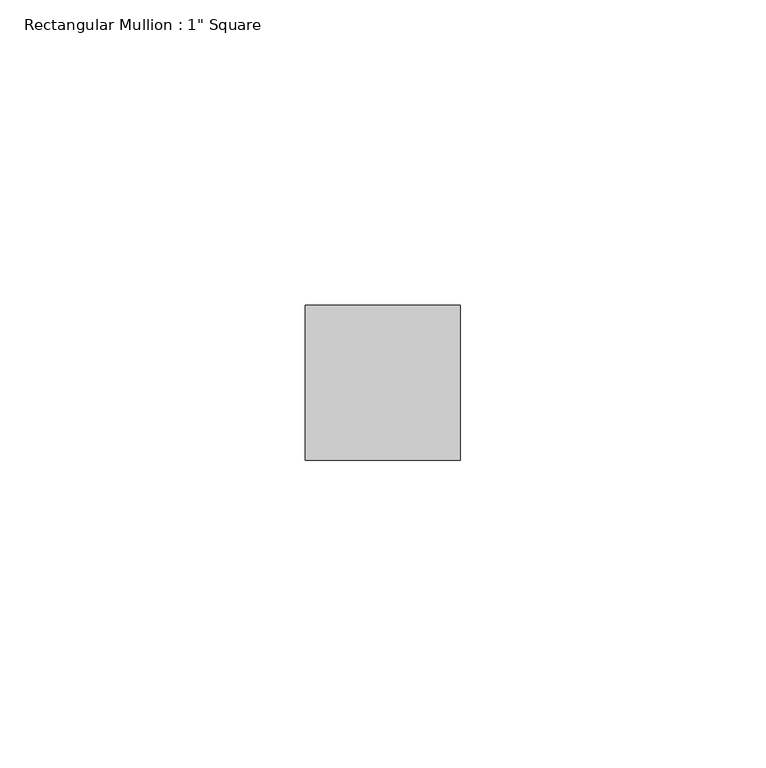
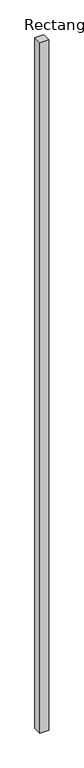
"""IFC4 building model written with IfcOpenShell, lengths in millimetres: member geometry."""

from ifc_helpers import new_model, si_unit, frame, origin, place, context, project, spatial, polyline, outline, extrude, source, transform, mapped, element, save


def member_dd05f1c1(model_context):
    return source(origin(), model_context, "Body", "SweptSolid", [
        extrude(outline(polyline([(0.0, 12.7), (0.0, -12.7), (-25.4, -12.7), (-25.4, 12.7), (0.0, 12.7)])), frame((0.0, 0.0, -2133.6), z_axis=(0.0, 0.0, 1.0), x_axis=(1.0, 0.0, 0.0)), (0.0, 0.0, 1.0), 2133.6),
    ])


if __name__ == "__main__":
    model = new_model("IFC4")
    model_context = context("Model", 3, world=origin())
    ifc_project = project(units=[si_unit("LENGTHUNIT", "METRE", prefix="MILLI")], contexts=[model_context])
    site = spatial("IfcSite", under=ifc_project)
    building = spatial("IfcBuilding", under=site)
    placement = place(None, origin())
    member_shape = member_dd05f1c1(model_context)
    element("IfcMember", 1, ObjectType="Rectangular Mullion : 1\" Square", at=placement, inside=building, context=model_context, shape_type="MappedRepresentation", body=[
        mapped(member_shape, transform((0.0, 0.0, 0.0), x_axis=(1.0, 0.0, 0.0), y_axis=(0.0, 1.0, 0.0), z_axis=(0.0, 0.0, 1.0))),
    ])
    save(model, "model.ifc")

# Revit data of these elements
# Type "Rectangular Mullion : 1\" Square"
#   built-in parameter 1007304 = 0.0833333 (stored number, unit not read)
#   built-in parameter 1007301 = 0.0416667 (stored number, unit not read)
#   built-in parameter 1007300 = 0.0416667 (stored number, unit not read)
# Element 1 (IfcMember, "Rectangular Mullion : 1\" Square")
#   Materials on its faces: "Aluminum"
# Materials
#   "Aluminum": class "Metal", colour RGB 247 247 247, transparency 0, Description = "Aluminum 6061", Cost = 0
